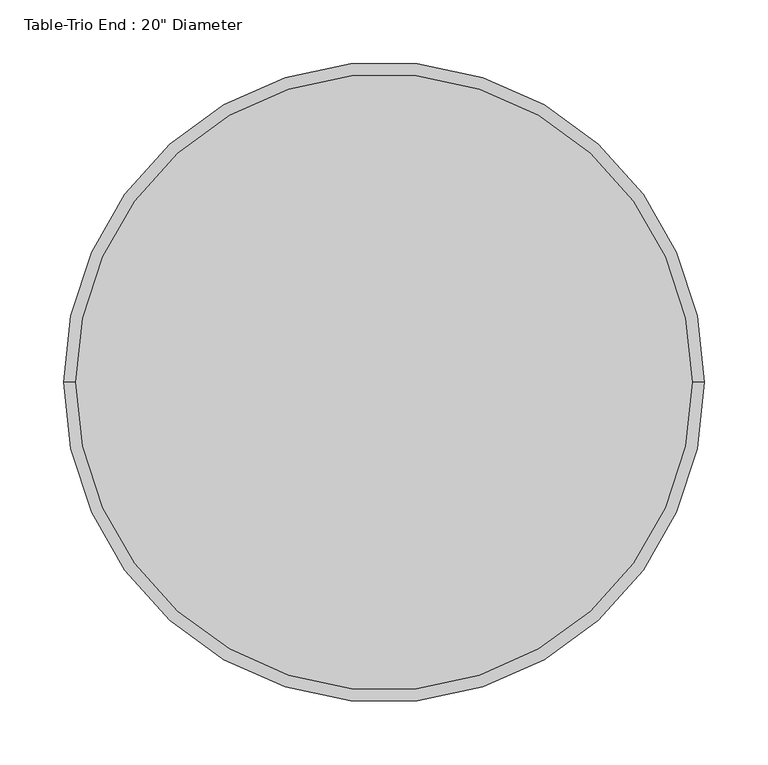
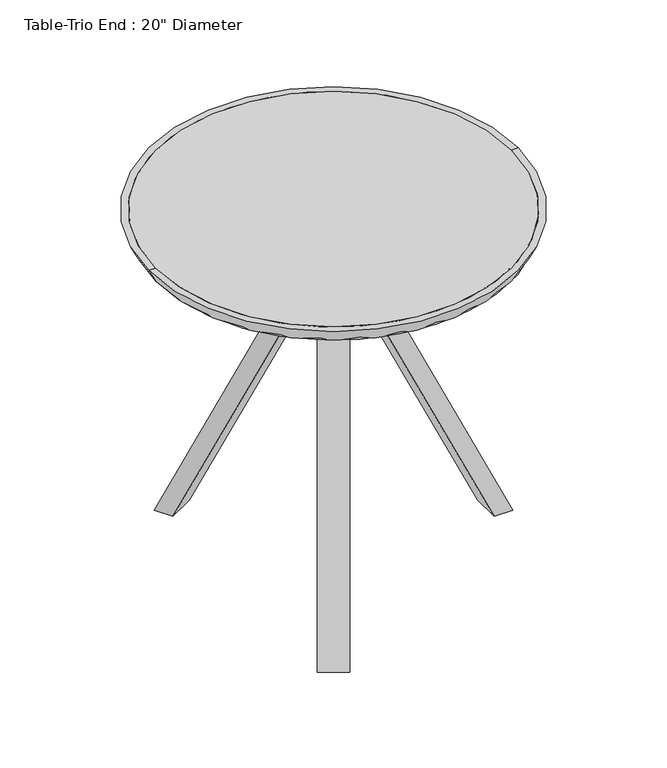
"""IFC4 building model written with IfcOpenShell, lengths in millimetres: furniture geometry."""

from ifc_helpers import new_model, si_unit, point, frame, frame_2d, origin, origin_2d, place, context, project, spatial, polyline, circle_curve, trimmed, segment, composite_curve, outline, extrude, source, transform, mapped, element, save
from ifc_brep_helpers import plane_surface, revolved_surface, advanced_brep


def furniture_9d41381f(model_context):
    return source(origin(), model_context, "Body", "SolidModel", [
        extrude(outline(composite_curve([segment(trimmed(circle_curve(origin_2d(), 241.3), [point((-241.3, 0.0))], [point((241.3, 0.0))], False, "CARTESIAN"), True, "CONTINUOUS"), segment(trimmed(circle_curve(origin_2d(), 241.3), [point((241.3, 0.0))], [point((-241.3, 0.0))], False, "CARTESIAN"), True, "CONTINUOUS")], self_intersect=False)), frame((0.0, 0.0, 482.6), z_axis=(0.0, 0.0, 1.0), x_axis=(1.0, 0.0, 0.0)), (0.0, 0.0, 1.0), 19.05),
        advanced_brep(
        [(241.3, 0.0, 482.6), (-241.3, 0.0, 482.6), (-241.3, 0.0, 501.65), (241.3, 0.0, 501.65), (250.825, 0.0, 501.65), (-250.825, 0.0, 501.65)],
        [
            (0, 1, circle_curve(frame((0.0, 0.0, 482.6), z_axis=(0.0, 0.0, -1.0), x_axis=(-1.0, 0.0, 0.0)), 241.3)),
            (1, 2),
            (2, 3, circle_curve(frame((0.0, 0.0, 501.65), z_axis=(0.0, 0.0, 1.0), x_axis=(-1.0, 0.0, 0.0)), 241.3)),
            (3, 0),
            (4, 5, circle_curve(frame((0.0, 0.0, 501.65), z_axis=(0.0, 0.0, -1.0), x_axis=(-1.0, 0.0, 0.0)), 250.825)),
            (5, 1),
            (0, 4),
            (2, 5),
            (4, 3),
            (1, 0, circle_curve(frame((0.0, 0.0, 482.6), z_axis=(0.0, 0.0, -1.0), x_axis=(1.0, 0.0, 0.0)), 241.3)),
            (3, 2, circle_curve(frame((0.0, 0.0, 501.65), z_axis=(0.0, 0.0, 1.0), x_axis=(1.0, 0.0, 0.0)), 241.3)),
            (5, 4, circle_curve(frame((0.0, 0.0, 501.65), z_axis=(0.0, 0.0, -1.0), x_axis=(1.0, 0.0, 0.0)), 250.825)),
        ],
        [
            revolved_surface(polyline([(-241.3, 0.0, 501.65), (-241.3, 0.0, 482.6)]), (0.0, 0.0, 0.0), (0.0, 0.0, 1.0)),
            revolved_surface(polyline([(-241.3, 0.0, 482.6), (-250.825, 0.0, 501.65)]), (0.0, 0.0, 0.0), (0.0, 0.0, 1.0)),
            plane_surface(frame((0.0, 0.0, 501.65), z_axis=(0.0, 0.0, 1.0), x_axis=(-1.0, 0.0, 0.0))),
            revolved_surface(polyline([(241.3, 0.0, 501.65), (241.3, 0.0, 482.6)]), (0.0, 0.0, 0.0), (0.0, 0.0, 1.0)),
            revolved_surface(polyline([(241.3, 0.0, 482.6), (250.825, 0.0, 501.65)]), (0.0, 0.0, 0.0), (0.0, 0.0, 1.0)),
            plane_surface(frame((0.0, 0.0, 501.65), z_axis=(0.0, 0.0, 1.0), x_axis=(1.0, 0.0, 0.0))),
        ],
        [
            (0, [[1, 2, 3, 4]]),
            (1, [[5, 6, -1, 7]]),
            (2, [[-3, 8, -5, 9]]),
            (3, [[10, -4, 11, -2]]),
            (4, [[12, -7, -10, -6]]),
            (5, [[-11, -9, -12, -8]]),
        ],
    ),
        extrude(outline(composite_curve([segment(polyline([(374.1964885, 32.5393466), (0.0, 207.0300348), (0.0, 232.3753669), (384.9309923, 52.8790974)]), True, "CONTINUOUS"), segment(trimmed(circle_curve(frame_2d((406.4, 98.9195329)), 50.8), [point((384.9309923, 52.8790974))], [point((457.2, 98.9195329))], True, "CARTESIAN"), True, "CONTINUOUS"), segment(polyline([(457.2, 98.9195329), (457.2, 154.8312035), (482.6, 154.8312035), (482.6, 101.6)]), True, "CONTINUOUS"), segment(trimmed(circle_curve(frame_2d((406.4, 101.6)), 76.2), [point((482.6, 101.6))], [point((374.1964885, 32.5393466))], False, "CARTESIAN"), True, "CONTINUOUS")], self_intersect=False)), frame((0.0, -19.05, 0.0), z_axis=(0.0, 1.0, 0.0), x_axis=(0.0, 0.0, 1.0)), (0.0, 0.0, 1.0), 38.1),
        extrude(outline(composite_curve([segment(trimmed(circle_curve(frame_2d((412.8801427, -76.2)), 76.2), [point((412.8801427, 0.0))], [point((481.9407961, -108.4035115))], False, "CARTESIAN"), True, "CONTINUOUS"), segment(polyline([(481.9407961, -108.4035115), (459.4443174, -156.6473658), (436.4240996, -145.9128619), (460.0533926, -95.2396796)]), True, "CONTINUOUS"), segment(trimmed(circle_curve(frame_2d((414.012957, -73.7706719)), 50.8), [point((460.0533926, -95.2396796))], [point((414.0129571, -22.9706718))], True, "CARTESIAN"), True, "CONTINUOUS"), segment(polyline([(414.0129571, -22.9706718), (-10.7114002, -22.9706719), (0.0, 0.0), (412.8801427, 0.0)]), True, "CONTINUOUS")], self_intersect=False)), frame((-120.0128014, 169.7682695, 0.0), z_axis=(0.8660254037844397, 0.4999999999999983, 0.0), x_axis=(0.2113091308703442, -0.36599815077065895, 0.9063077870366545)), (0.0, 0.0, 1.0), 38.1),
        extrude(outline(composite_curve([segment(trimmed(circle_curve(frame_2d((412.8801427, -76.2)), 76.2), [point((412.8801427, 0.0))], [point((481.9407961, -108.4035116))], False, "CARTESIAN"), True, "CONTINUOUS"), segment(polyline([(481.9407961, -108.4035116), (459.4443174, -156.6473658), (436.4240996, -145.9128619), (460.0533926, -95.2396796)]), True, "CONTINUOUS"), segment(trimmed(circle_curve(frame_2d((414.012957, -73.7706719)), 50.8), [point((460.0533926, -95.2396796))], [point((414.0129571, -22.9706718))], True, "CARTESIAN"), True, "CONTINUOUS"), segment(polyline([(414.0129571, -22.9706718), (-10.7114002, -22.9706719), (0.0, 0.0), (412.8801427, 0.0)]), True, "CONTINUOUS")], self_intersect=False)), frame((-87.0172335, -188.8182695, 0.0), z_axis=(-0.8660254037844366, 0.5000000000000038, 0.0), x_axis=(0.21130913087034656, 0.3659981507706578, 0.9063077870366544)), (0.0, 0.0, 1.0), 38.1),
        extrude(outline(composite_curve([segment(trimmed(circle_curve(origin_2d(), 31.7871474), [point((-31.7871474, 0.0))], [point((31.7871474, 0.0))], False, "CARTESIAN"), True, "CONTINUOUS"), segment(trimmed(circle_curve(origin_2d(), 31.7871474), [point((31.7871474, 0.0))], [point((-31.7871474, 0.0))], False, "CARTESIAN"), True, "CONTINUOUS")], self_intersect=False)), frame((0.0, 0.0, 381.0), z_axis=(0.0, 0.0, 1.0), x_axis=(1.0, 0.0, 0.0)), (0.0, 0.0, 1.0), 50.8),
    ])


if __name__ == "__main__":
    model = new_model("IFC4")
    model_context = context("Model", 3, world=origin())
    ifc_project = project(units=[si_unit("LENGTHUNIT", "METRE", prefix="MILLI")], contexts=[model_context])
    site = spatial("IfcSite", under=ifc_project)
    building = spatial("IfcBuilding", under=site)
    placement = place(None, origin())
    furniture_shape = furniture_9d41381f(model_context)
    element("IfcFurniture", 1, ObjectType="Table-Trio End : 20\" Diameter", at=placement, inside=building, context=model_context, shape_type="MappedRepresentation", body=[
        mapped(furniture_shape, transform((0.0, 0.0, 0.0), x_axis=(1.0, 0.0, 0.0), y_axis=(0.0, 1.0, 0.0), z_axis=(0.0, 0.0, 1.0))),
    ])
    save(model, "model.ifc")

# Revit data of these elements
# Type "Table-Trio End : 20\" Diameter"
#   Assembly Code = "E2020200"
#   Base and Trim Material = Wood - Birch
#   Table Top Material = Laminate - Ivory,Matte
#   Default Elevation = 0
# Element 1 (IfcFurniture, "Table-Trio End : 20\" Diameter")
#   Materials on its faces: "Wood - Birch", "Laminate - Ivory,Matte"
# Materials
#   "Wood - Birch": colour RGB 230 196 162, transparency 0
#   "Laminate - Ivory,Matte": colour RGB 127 127 127, transparency 0
